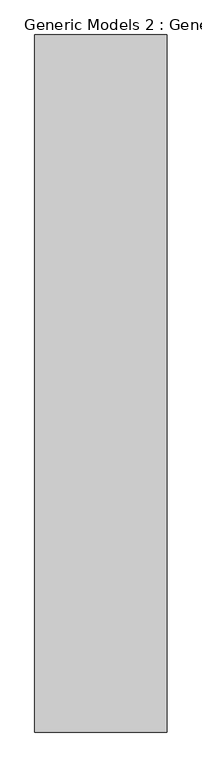
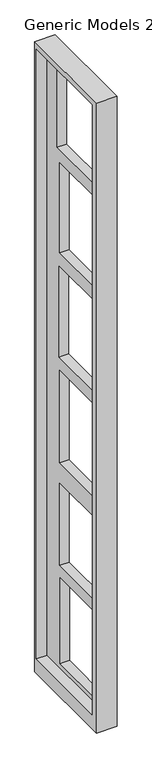
"""IFC4 building model written with IfcOpenShell, lengths in millimetres: proxy geometry, Generic Models 2 : Generic Models 1."""

from ifc_helpers import new_model, si_unit, origin, place, context, project, spatial, faceted_brep, source, transform, mapped, element, save


def generic_models_2_generic_models_1_16343201(model_context):
    return source(origin(), model_context, "Body", "Brep", [
        faceted_brep([(-6457.5487703, -529.1037749, 18288.0), (-6457.5487703, 2442.6962251, 18288.0), (-7022.5256993, 2442.6962251, 18288.0), (-7022.5256993, -529.1037749, 18288.0), (-6457.5487703, -529.1037749, -158.4213758), (-7022.5256993, -529.1037749, -158.4213758), (-7022.5256993, 2442.6962251, -158.4213758), (-6457.5487703, 2442.6962251, -158.4213758), (-6457.5487703, 80.4962251, 15427.4465317), (-6457.5487703, 80.4962251, 17896.0910797), (-6457.5487703, 1889.1429371, 17896.0910797), (-6457.5487703, 1889.1429371, 15427.4465317), (-6457.5487703, -8.6872134, 12397.0580072), (-6457.5487703, -8.6872134, 15042.3231805), (-6457.5487703, 1781.5076359, 15042.3231805), (-6457.5487703, 1781.5076359, 12397.0580072), (-6457.5487703, -17.3853235, 9328.6434489), (-6457.5487703, -17.3853235, 11990.9234937), (-6457.5487703, 1807.8390259, 11990.9234937), (-6457.5487703, 1807.8390259, 9328.6434489), (-6457.5487703, -30.6801441, 6248.4), (-6457.5487703, -30.6801441, 8955.1024994), (-6457.5487703, 1778.1125113, 8955.1024994), (-6457.5487703, 1778.1125113, 6248.4), (-6457.5487703, -22.1772395, 3249.0844472), (-6457.5487703, -22.1772395, 5661.4894523), (-6457.5487703, 1769.7396662, 5661.4894523), (-6457.5487703, 1769.7396662, 3249.0844472), (-6457.5487703, -35.8456262, 382.1575328), (-6457.5487703, -35.8456262, 2893.6398867), (-6457.5487703, 1759.3912226, 2893.6398867), (-6457.5487703, 1759.3912226, 382.1575328), (-7022.5256993, -312.6392341, 18107.7487565), (-7022.5256993, -312.6392341, 247.1582995), (-7022.5256993, 2381.9388528, 247.1582995), (-7022.5256993, 2381.9388528, 18107.7487565), (-6717.7256993, -312.6392341, 18107.7487565), (-6717.7256993, 2381.9388528, 18107.7487565), (-6717.7256993, 2381.9388528, 247.1582995), (-6717.7256993, -312.6392341, 247.1582995), (-6717.7256993, 80.4962251, 17896.0910797), (-6717.7256993, 80.4962251, 15427.4465317), (-6717.7256993, 1889.1429371, 15427.4465317), (-6717.7256993, 1889.1429371, 17896.0910797), (-6717.7256993, -8.6872134, 15042.3231805), (-6717.7256993, -8.6872134, 12397.0580072), (-6717.7256993, 1781.5076359, 12397.0580072), (-6717.7256993, 1781.5076359, 15042.3231805), (-6717.7256993, -17.3853235, 11990.9234937), (-6717.7256993, -17.3853235, 9328.6434489), (-6717.7256993, 1807.8390259, 9328.6434489), (-6717.7256993, 1807.8390259, 11990.9234937), (-6717.7256993, -30.6801441, 8955.1024994), (-6717.7256993, -30.6801441, 6248.4), (-6717.7256993, 1778.1125113, 6248.4), (-6717.7256993, 1778.1125113, 8955.1024994), (-6717.7256993, -22.1772395, 5661.4894523), (-6717.7256993, -22.1772395, 3249.0844472), (-6717.7256993, 1769.7396662, 3249.0844472), (-6717.7256993, 1769.7396662, 5661.4894523), (-6717.7256993, -35.8456262, 2893.6398867), (-6717.7256993, -35.8456262, 382.1575328), (-6717.7256993, 1759.3912226, 382.1575328), (-6717.7256993, 1759.3912226, 2893.6398867)], [[[0, 1, 2, 3]], [[4, 5, 6, 7]], [[1, 0, 4, 7], [8, 9, 10, 11], [12, 13, 14, 15], [16, 17, 18, 19], [20, 21, 22, 23], [24, 25, 26, 27], [28, 29, 30, 31]], [[2, 1, 7, 6]], [[3, 2, 6, 5], [32, 33, 34, 35]], [[0, 3, 5, 4]], [[36, 37, 38, 39], [40, 41, 42, 43], [44, 45, 46, 47], [48, 49, 50, 51], [52, 53, 54, 55], [56, 57, 58, 59], [60, 61, 62, 63]], [[36, 39, 33, 32]], [[39, 38, 34, 33]], [[38, 37, 35, 34]], [[37, 36, 32, 35]], [[40, 9, 8, 41]], [[41, 8, 11, 42]], [[42, 11, 10, 43]], [[9, 40, 43, 10]], [[44, 13, 12, 45]], [[45, 12, 15, 46]], [[46, 15, 14, 47]], [[13, 44, 47, 14]], [[48, 17, 16, 49]], [[49, 16, 19, 50]], [[50, 19, 18, 51]], [[17, 48, 51, 18]], [[52, 21, 20, 53]], [[53, 20, 23, 54]], [[54, 23, 22, 55]], [[21, 52, 55, 22]], [[56, 25, 24, 57]], [[57, 24, 27, 58]], [[58, 27, 26, 59]], [[25, 56, 59, 26]], [[60, 29, 28, 61]], [[61, 28, 31, 62]], [[62, 31, 30, 63]], [[29, 60, 63, 30]]]),
    ])


if __name__ == "__main__":
    model = new_model("IFC4")
    model_context = context("Model", 3, world=origin())
    ifc_project = project(units=[si_unit("LENGTHUNIT", "METRE", prefix="MILLI")], contexts=[model_context])
    site = spatial("IfcSite", under=ifc_project)
    building = spatial("IfcBuilding", under=site)
    placement = place(None, origin())
    generic_models_2_generic_models_1_shape = generic_models_2_generic_models_1_16343201(model_context)
    element("IfcBuildingElementProxy", 1, Name="Generic Models 2 : Generic Models 1", ObjectType="Generic Models 2 : Generic Models 1", at=placement, inside=building, context=model_context, shape_type="MappedRepresentation", body=[
        mapped(generic_models_2_generic_models_1_shape, transform((0.0, 0.0, 0.0), x_axis=(1.0, 0.0, 0.0), y_axis=(0.0, 1.0, 0.0), z_axis=(0.0, 0.0, 1.0))),
    ])
    save(model, "model.ifc")
